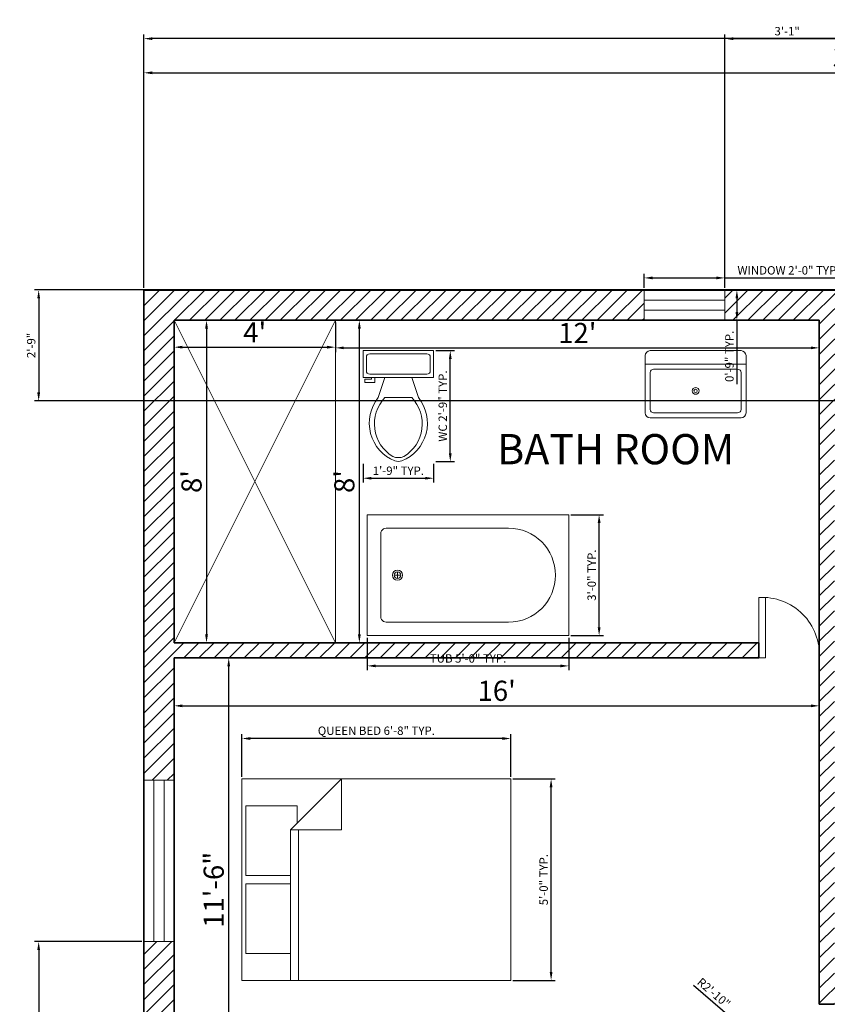
# Model space of a CAD drawing. Units: inches. Extents: x 4740 to 5323, y 7115 to 7713.
# Tile 3 of 6: x 4740 to 4980, y 7420 to 7713. Entities that reach past the tile are written whole.
import ezdxf

# ---------------------------------------------------------------- set-up
doc = ezdxf.new("R2010")
doc.units = ezdxf.units.IN
for name, color, linetype, lineweight in [('A-ANNO-DIMS', 2, 'Continuous', 18), ('A-AREA-IDEN', 7, 'Continuous', 25), ('A-DOOR', 4, 'Continuous', 18), ('A-FLOR-FIXT', 9, 'Continuous', 18), ('A-FURN', 8, 'Continuous', 18), ('A-GLAZ', 242, 'Continuous', 18), ('A-WALL', 7, 'Continuous', 35)]:
    doc.layers.add(name, color=color, linetype=linetype, lineweight=lineweight)
doc.layers.add('A-WALL-PATT', color=152, linetype='Continuous', lineweight=13, true_color=0x2776bb)
doc.styles.get("Standard").update_dxf_attribs({"font": 'arial.ttf'})
doc.dimstyles.new('ISO-25', dxfattribs={"dimtxt": 2.5, "dimasz": 2.5, "dimexe": 1.25, "dimexo": 0.625, "dimtad": 1, "dimlunit": 3, "dimtxsty": 'Standard', "dimcen": 2.5, "dimadec": 0, "dimazin": 0, "dimtfac": 1, "dimtmove": 0, "dimatfit": 3, "dimfxl": 1, "dimarcsym": 0})

# ---------------------------------------------------------------- blocks, each defined once
blk = doc.blocks.new('*D11')
at = {"layer": 'A-ANNO-DIMS', "color": 0, "lineweight": -2, "transparency": 16777216}
for p, q in [((4785.46, 7622.73), (4785.46, 7614.09)), ((4833.46, 7622.73), (4833.46, 7614.09)), ((4787.96, 7615.34), (4830.96, 7615.34))]:
    blk.add_line(p, q, dxfattribs=at)
at = {"layer": 'A-ANNO-DIMS', "color": 0, "transparency": 16777216}
for points in [[(4787.96, 7615.76), (4787.96, 7614.92), (4785.46, 7615.34)], [(4830.96, 7615.76), (4830.96, 7614.92), (4833.46, 7615.34)]]:
    blk.add_solid(points, dxfattribs=at)
at = {"layer": 'Defpoints', "color": 0, "transparency": 16777216}
for p in [(4785.46, 7623.36), (4833.46, 7623.36), (4833.46, 7615.34)]:
    blk.add_point(p, dxfattribs=at)
at = {"layer": 'A-ANNO-DIMS', "color": 0, "transparency": 16777216, "insert": (4809.46, 7618.97), "char_height": 6, "attachment_point": 5}
blk.add_mtext("4'", dxfattribs=at)
blk = doc.blocks.new('*D12')
at = {"layer": 'A-ANNO-DIMS', "color": 0, "lineweight": -2, "transparency": 16777216}
for p, q in [((4786.08, 7623.36), (4796.37, 7623.36)), ((4795.12, 7620.86), (4795.12, 7529.86)), ((4786.08, 7527.36), (4796.37, 7527.36))]:
    blk.add_line(p, q, dxfattribs=at)
at = {"layer": 'A-ANNO-DIMS', "color": 0, "transparency": 16777216}
for points in [[(4794.7, 7620.86), (4795.54, 7620.86), (4795.12, 7623.36)], [(4794.7, 7529.86), (4795.54, 7529.86), (4795.12, 7527.36)]]:
    blk.add_solid(points, dxfattribs=at)
at = {"layer": 'Defpoints', "color": 0, "transparency": 16777216}
for p in [(4785.46, 7623.36), (4785.46, 7527.36), (4795.12, 7527.36)]:
    blk.add_point(p, dxfattribs=at)
at = {"layer": 'A-ANNO-DIMS', "color": 0, "transparency": 16777216, "insert": (4791.43, 7575.36), "char_height": 6, "attachment_point": 5, "rotation": 90}
blk.add_mtext("8'", dxfattribs=at)
blk = doc.blocks.new('*D13')
at = {"layer": 'A-ANNO-DIMS', "color": 0, "lineweight": -2, "transparency": 16777216}
for p, q in [((4834.08, 7623.36), (4841.84, 7623.36)), ((4840.59, 7529.86), (4840.59, 7620.86)), ((4834.08, 7527.36), (4841.84, 7527.36))]:
    blk.add_line(p, q, dxfattribs=at)
at = {"layer": 'A-ANNO-DIMS', "color": 0, "transparency": 16777216}
for points in [[(4840.18, 7620.86), (4841.01, 7620.86), (4840.59, 7623.36)], [(4840.18, 7529.86), (4841.01, 7529.86), (4840.59, 7527.36)]]:
    blk.add_solid(points, dxfattribs=at)
at = {"layer": 'Defpoints', "color": 0, "transparency": 16777216}
for p in [(4833.46, 7623.36), (4840.59, 7623.36), (4833.46, 7527.36)]:
    blk.add_point(p, dxfattribs=at)
at = {"layer": 'A-ANNO-DIMS', "color": 0, "transparency": 16777216, "insert": (4836.9, 7575.36), "char_height": 6, "attachment_point": 5, "rotation": 90}
blk.add_mtext("8'", dxfattribs=at)
blk = doc.blocks.new('*D14')
at = {"layer": 'A-ANNO-DIMS', "color": 0, "lineweight": -2, "transparency": 16777216}
for p, q in [((4833.46, 7622.73), (4833.46, 7613.89)), ((4977.46, 7622.73), (4977.46, 7613.89)), ((4835.96, 7615.14), (4974.96, 7615.14))]:
    blk.add_line(p, q, dxfattribs=at)
at = {"layer": 'A-ANNO-DIMS', "color": 0, "transparency": 16777216}
for points in [[(4835.96, 7615.55), (4835.96, 7614.72), (4833.46, 7615.14)], [(4974.96, 7615.55), (4974.96, 7614.72), (4977.46, 7615.14)]]:
    blk.add_solid(points, dxfattribs=at)
at = {"layer": 'Defpoints', "color": 0, "transparency": 16777216}
for p in [(4833.46, 7623.36), (4977.46, 7623.36), (4977.46, 7615.14)]:
    blk.add_point(p, dxfattribs=at)
at = {"layer": 'A-ANNO-DIMS', "color": 0, "transparency": 16777216, "insert": (4905.46, 7618.77), "char_height": 6, "width": 4.0075, "attachment_point": 5}
blk.add_mtext("12'", dxfattribs=at)
blk = doc.blocks.new('*D15')
at = {"layer": 'A-ANNO-DIMS', "color": 0, "lineweight": -2, "transparency": 16777216}
for p, q in [((4785.46, 7522.23), (4785.46, 7507.36)), ((4977.46, 7522.23), (4977.46, 7507.36)), ((4787.96, 7508.61), (4974.96, 7508.61))]:
    blk.add_line(p, q, dxfattribs=at)
at = {"layer": 'A-ANNO-DIMS', "color": 0, "transparency": 16777216}
for points in [[(4787.96, 7509.02), (4787.96, 7508.19), (4785.46, 7508.61)], [(4974.96, 7509.02), (4974.96, 7508.19), (4977.46, 7508.61)]]:
    blk.add_solid(points, dxfattribs=at)
at = {"layer": 'Defpoints', "color": 0, "transparency": 16777216}
for p in [(4785.46, 7522.86), (4977.46, 7522.86), (4977.46, 7508.61)]:
    blk.add_point(p, dxfattribs=at)
at = {"layer": 'A-ANNO-DIMS', "color": 0, "transparency": 16777216, "insert": (4881.46, 7512.3), "char_height": 6, "attachment_point": 5}
blk.add_mtext("16'", dxfattribs=at)
blk = doc.blocks.new('*D16')
at = {"layer": 'A-ANNO-DIMS', "color": 0, "lineweight": -2, "transparency": 16777216}
for p, q in [((4786.08, 7522.86), (4802.97, 7522.86)), ((4801.72, 7387.36), (4801.72, 7520.36)), ((4786.08, 7384.86), (4802.97, 7384.86))]:
    blk.add_line(p, q, dxfattribs=at)
at = {"layer": 'A-ANNO-DIMS', "color": 0, "transparency": 16777216}
for points in [[(4801.3, 7520.36), (4802.13, 7520.36), (4801.72, 7522.86)], [(4801.3, 7387.36), (4802.13, 7387.36), (4801.72, 7384.86)]]:
    blk.add_solid(points, dxfattribs=at)
at = {"layer": 'Defpoints', "color": 0, "transparency": 16777216}
for p in [(4785.46, 7522.86), (4801.72, 7522.86), (4785.46, 7384.86)]:
    blk.add_point(p, dxfattribs=at)
at = {"layer": 'A-ANNO-DIMS', "color": 0, "transparency": 16777216, "insert": (4798.03, 7453.86), "char_height": 6, "attachment_point": 5, "rotation": 90}
blk.add_mtext('11\'-6"', dxfattribs=at)
blk = doc.blocks.new('Bath Tub - 26 x 60 in.')
for p, q in [((9, -17), (9, -19)), ((8, -18), (10, -18))]:
    blk.add_line(p, q)
blk.add_lwpolyline([(0, -36), (0, 0), (60, 0), (60, -36)], close=True)
for points in [[(6, -4), (42, -4)], [(4, -30), (4, -6)], [(42, -32), (6, -32)]]:
    blk.add_lwpolyline(points)
for radius in [1.5, 1]:
    blk.add_circle((9, -18), radius)
for centre, radius, start, end in [((5.75, -5.75), 1.77, 81.8699, 188.1301), ((42, -18), 14, 270, 90), ((5.75, -30.25), 1.77, 171.8699, 278.1301)]:
    blk.add_arc(centre, radius, start, end)
blk = doc.blocks.new('Toilet - top')
for p, q in [((9.5, -6), (9.5, -2)), ((-10, -8.5), (-8, -8.5)), ((-10, -9.5), (-10, -8.5)), ((-8, -8.5), (-8, -8)), ((-7, -8), (-7, -9.5)), ((-4, -8), (-6, -14)), ((4, -8), (6, -14)), ((-7, -9.5), (-10, -9.5)), ((4, -14), (-4, -14))]:
    blk.add_line(p, q)
blk.add_lwpolyline([(10.5, -8), (10.5, 0), (-10.5, 0), (-10.5, -8)], close=True)
for points in [[(-9.5, -2), (-9.5, -6)], [(8.5, -1), (-8.5, -1)], [(-8.5, -7), (8.5, -7)]]:
    blk.add_lwpolyline(points)
for centre, radius, start, end in [((-8.62, -1.88), 0.884, 81.8699, 188.1301), ((8.62, -1.88), 0.884, 351.8699, 98.1301), ((-8.62, -6.12), 0.884, 171.8699, 278.1301), ((8.62, -6.12), 0.884, 261.8699, 8.1301), ((3.52, -21.58), 12.17, 141.4691, 247.9714), ((4.2, -21.82), 11.33, 136.3677, 238.9468), ((-3.52, -21.58), 12.17, 292.0284, 38.5307), ((-4.2, -21.82), 11.33, 301.053, 43.6321), ((0, -27.88), 4, 245.7318, 294.2682), ((0, -29), 4, 254.8605, 285.1395)]:
    blk.add_arc(centre, radius, start, end)
blk = doc.blocks.new('Bed - Queen')
for p, q in [((0, -80.00003), (0, 0)), ((0, 0), (59.99999, 0)), ((59.99999, 0), (59.99999, -80.00003)), ((7.99999, -1.2), (28.79998, -1.2)), ((7.99999, -14.4), (7.99999, -1.2)), ((28.79998, -1.2), (28.79998, -14.4)), ((31.19999, -1.2), (51.99999, -1.2)), ((31.19999, -14.4), (31.19999, -1.2)), ((51.99999, -1.2), (51.99999, -16.4)), ((0, -14.4), (44.8, -14.4)), ((59.99999, -29.6), (44.8, -14.4)), ((44.8, -14.4), (44.8, -29.6)), ((44.8, -16.8), (0, -16.8)), ((51.99999, -16.4), (46.79936, -16.4)), ((44.8, -29.6), (59.99999, -29.6)), ((59.99999, -80.00003), (0, -80.00003))]:
    blk.add_line(p, q)
blk = doc.blocks.new('Sink-single - 30 in top')
blk.add_line((-15, -3.999996), (15, -3.999996))
for points in [[(-13.5, 0), (13.5, 0)], [(-15, -18.499996), (-15, -1.5)], [(15, -1.5), (15, -18.499996)], [(-12.5, -5.499996), (12.5, -5.499996)], [(-13.5, -17.499996), (-13.5, -6.499996)], [(13.5, -6.499996), (13.5, -17.499996)], [(13.5, -19.999996), (-13.5, -19.999996)], [(12.5, -18.499996), (-12.5, -18.499996)]]:
    blk.add_lwpolyline(points)
for radius in [1, 0.5]:
    blk.add_circle((0, -11.999996), radius)
for centre, radius, start, end in [((-13.5, -1.5), 1.5, 90, 180), ((13.5, -1.5), 1.5, 0, 90), ((-12.5, -6.499996), 1, 90, 180), ((12.5, -6.499996), 1, 0, 90), ((-12.5, -17.499996), 1, 180, 270), ((12.5, -17.499996), 1, 270, 0), ((-13.5, -18.499996), 1.5, 180, 270), ((13.5, -18.499996), 1.5, 270, 0)]:
    blk.add_arc(centre, radius, start, end)
blk = doc.blocks.new('*D35')
at = {"layer": 'A-ANNO-DIMS', "color": 0, "lineweight": -2, "transparency": 16777216}
for p, q in [((4776.46, 7632.98), (4776.46, 7698.25)), ((5215.96, 7629.25), (5215.96, 7698.25)), ((4778.96, 7697), (5213.46, 7697))]:
    blk.add_line(p, q, dxfattribs=at)
at = {"layer": 'A-ANNO-DIMS', "color": 0, "transparency": 16777216}
for points in [[(4778.96, 7697.42), (4778.96, 7696.58), (4776.46, 7697)], [(5213.46, 7697.42), (5213.46, 7696.58), (5215.96, 7697)]]:
    blk.add_solid(points, dxfattribs=at)
at = {"layer": 'Defpoints', "color": 0, "transparency": 16777216}
for p in [(5215.96, 7697), (4776.46, 7632.36), (5215.96, 7628.62)]:
    blk.add_point(p, dxfattribs=at)
at = {"layer": 'A-ANNO-DIMS', "color": 0, "transparency": 16777216, "insert": (4996.21, 7700.69), "char_height": 6, "attachment_point": 5}
blk.add_mtext('36\'-7.5"', dxfattribs=at)
blk = doc.blocks.new('WIN-48IN')
for p, q in [((0, 0), (0, 9)), ((0, 9), (48, 9)), ((48, 9), (48, 0)), ((0, 6), (48, 6)), ((0, 3), (48, 3)), ((48, 0), (0, 0))]:
    blk.add_line(p, q)
blk = doc.blocks.new('WIN-24IN')
for p, q in [((0, 24), (9, 24)), ((0, 24), (0, 0)), ((3, 0), (3, 24)), ((6, 0), (6, 24)), ((9, 0), (9, 24)), ((0, 0), (9, 0))]:
    blk.add_line(p, q)
blk = doc.blocks.new('DOOR-SWING-18IN')
for p, q in [((0, 0), (0, 18)), ((0, 18), (2, 18)), ((2, 18), (2, 0)), ((2, 0), (0, 0))]:
    blk.add_line(p, q)
blk.add_arc((1, 1), 17.03, 356.6335, 93.3665)
blk = doc.blocks.new('*D44')
at = {"layer": 'A-ANNO-DIMS', "color": 0, "lineweight": -2, "transparency": 16777216}
for p, q in [((4925.34, 7632.98), (4925.34, 7637.21)), ((4949.34, 7632.98), (4949.34, 7637.21)), ((4927.84, 7635.96), (4946.84, 7635.96)), ((4949.34, 7635.96), (4984.73, 7635.96))]:
    blk.add_line(p, q, dxfattribs=at)
at = {"layer": 'A-ANNO-DIMS', "color": 0, "transparency": 16777216}
for points in [[(4927.84, 7636.37), (4927.84, 7635.54), (4925.34, 7635.96)], [(4946.84, 7636.37), (4946.84, 7635.54), (4949.34, 7635.96)]]:
    blk.add_solid(points, dxfattribs=at)
at = {"layer": 'Defpoints', "color": 0, "transparency": 16777216}
for p in [(4949.34, 7635.96), (4925.34, 7632.36), (4949.34, 7632.36)]:
    blk.add_point(p, dxfattribs=at)
at = {"layer": 'A-ANNO-DIMS', "color": 0, "transparency": 16777216, "insert": (4968.29, 7637.88), "char_height": 2.5, "attachment_point": 5}
blk.add_mtext('WINDOW 2\'-0" TYP.', dxfattribs=at)
blk = doc.blocks.new('*D45')
at = {"layer": 'A-ANNO-DIMS', "color": 0, "lineweight": -2, "transparency": 16777216}
for p, q in [((4949.97, 7632.36), (4954.19, 7632.36)), ((4952.94, 7629.86), (4952.94, 7625.86)), ((4949.97, 7623.36), (4954.19, 7623.36)), ((4952.94, 7623.36), (4952.94, 7604.37))]:
    blk.add_line(p, q, dxfattribs=at)
at = {"layer": 'A-ANNO-DIMS', "color": 0, "transparency": 16777216}
for points in [[(4952.53, 7629.86), (4953.36, 7629.86), (4952.94, 7632.36)], [(4952.53, 7625.86), (4953.36, 7625.86), (4952.94, 7623.36)]]:
    blk.add_solid(points, dxfattribs=at)
at = {"layer": 'Defpoints', "color": 0, "transparency": 16777216}
for p in [(4949.34, 7632.36), (4949.34, 7623.36), (4952.94, 7623.36)]:
    blk.add_point(p, dxfattribs=at)
at = {"layer": 'A-ANNO-DIMS', "color": 0, "transparency": 16777216, "insert": (4951.04, 7612.61), "char_height": 2.5, "attachment_point": 5, "rotation": 90}
blk.add_mtext('0\'-9" TYP.', dxfattribs=at)
blk = doc.blocks.new('*D48')
at = {"layer": 'A-ANNO-DIMS', "color": 0, "lineweight": -2, "transparency": 16777216}
for p, q in [((4842.95, 7528.86), (4842.95, 7519.24)), ((4902.95, 7528.86), (4902.95, 7519.24)), ((4845.45, 7520.49), (4900.45, 7520.49))]:
    blk.add_line(p, q, dxfattribs=at)
at = {"layer": 'A-ANNO-DIMS', "color": 0, "transparency": 16777216}
for points in [[(4845.45, 7520.9), (4845.45, 7520.07), (4842.95, 7520.49)], [(4900.45, 7520.9), (4900.45, 7520.07), (4902.95, 7520.49)]]:
    blk.add_solid(points, dxfattribs=at)
at = {"layer": 'Defpoints', "color": 0, "transparency": 16777216}
for p in [(4842.95, 7529.49), (4902.95, 7529.49), (4902.95, 7520.49)]:
    blk.add_point(p, dxfattribs=at)
at = {"layer": 'A-ANNO-DIMS', "color": 0, "transparency": 16777216, "insert": (4872.95, 7522.39), "char_height": 2.5, "attachment_point": 5}
blk.add_mtext('TUB 5\'-0" TYP.', dxfattribs=at)
blk = doc.blocks.new('*D49')
at = {"layer": 'A-ANNO-DIMS', "color": 0, "lineweight": -2, "transparency": 16777216}
for p, q in [((4903.57, 7565.49), (4913.2, 7565.49)), ((4911.95, 7531.99), (4911.95, 7562.99)), ((4903.57, 7529.49), (4913.2, 7529.49))]:
    blk.add_line(p, q, dxfattribs=at)
at = {"layer": 'A-ANNO-DIMS', "color": 0, "transparency": 16777216}
for points in [[(4911.53, 7562.99), (4912.37, 7562.99), (4911.95, 7565.49)], [(4911.53, 7531.99), (4912.37, 7531.99), (4911.95, 7529.49)]]:
    blk.add_solid(points, dxfattribs=at)
at = {"layer": 'Defpoints', "color": 0, "transparency": 16777216}
for p in [(4902.95, 7565.49), (4911.95, 7565.49), (4902.95, 7529.49)]:
    blk.add_point(p, dxfattribs=at)
at = {"layer": 'A-ANNO-DIMS', "color": 0, "transparency": 16777216, "insert": (4910.05, 7547.49), "char_height": 2.5, "attachment_point": 5, "rotation": 90}
blk.add_mtext('3\'-0" TYP.', dxfattribs=at)
blk = doc.blocks.new('*D50')
at = {"layer": 'A-ANNO-DIMS', "color": 0, "lineweight": -2, "transparency": 16777216}
for p, q in [((4805.65, 7487.5), (4805.65, 7500.13)), ((4883.16, 7498.88), (4808.15, 7498.88)), ((4885.66, 7487.5), (4885.66, 7500.13))]:
    blk.add_line(p, q, dxfattribs=at)
at = {"layer": 'A-ANNO-DIMS', "color": 0, "transparency": 16777216}
for points in [[(4808.15, 7499.29), (4808.15, 7498.46), (4805.65, 7498.88)], [(4883.16, 7499.29), (4883.16, 7498.46), (4885.66, 7498.88)]]:
    blk.add_solid(points, dxfattribs=at)
at = {"layer": 'Defpoints', "color": 0, "transparency": 16777216}
for p in [(4805.65, 7498.88), (4805.65, 7486.88), (4885.66, 7486.88)]:
    blk.add_point(p, dxfattribs=at)
at = {"layer": 'A-ANNO-DIMS', "color": 0, "transparency": 16777216, "insert": (4845.65, 7500.87), "char_height": 2.5, "attachment_point": 5}
blk.add_mtext('QUEEN BED 6\'-8" TYP.', dxfattribs=at)
blk = doc.blocks.new('*D51')
at = {"layer": 'A-ANNO-DIMS', "color": 0, "lineweight": -2, "transparency": 16777216}
for p, q in [((4886.28, 7486.88), (4898.91, 7486.88)), ((4897.66, 7429.38), (4897.66, 7484.38)), ((4886.28, 7426.88), (4898.91, 7426.88))]:
    blk.add_line(p, q, dxfattribs=at)
at = {"layer": 'A-ANNO-DIMS', "color": 0, "transparency": 16777216}
for points in [[(4897.24, 7484.38), (4898.07, 7484.38), (4897.66, 7486.88)], [(4897.24, 7429.38), (4898.07, 7429.38), (4897.66, 7426.88)]]:
    blk.add_solid(points, dxfattribs=at)
at = {"layer": 'Defpoints', "color": 0, "transparency": 16777216}
for p in [(4885.66, 7486.88), (4897.66, 7486.88), (4885.66, 7426.88)]:
    blk.add_point(p, dxfattribs=at)
at = {"layer": 'A-ANNO-DIMS', "color": 0, "transparency": 16777216, "insert": (4895.75, 7456.88), "char_height": 2.5, "attachment_point": 5, "rotation": 90}
blk.add_mtext('5\'-0" TYP.', dxfattribs=at)
blk = doc.blocks.new('*D52')
at = {"layer": 'A-ANNO-DIMS', "color": 0, "lineweight": -2, "transparency": 16777216}
for p, q in [((4863.32, 7614.34), (4868.9, 7614.34)), ((4867.65, 7583.79), (4867.65, 7611.84)), ((4863.32, 7581.29), (4868.9, 7581.29))]:
    blk.add_line(p, q, dxfattribs=at)
at = {"layer": 'A-ANNO-DIMS', "color": 0, "transparency": 16777216}
for points in [[(4867.24, 7611.84), (4868.07, 7611.84), (4867.65, 7614.34)], [(4867.24, 7583.79), (4868.07, 7583.79), (4867.65, 7581.29)]]:
    blk.add_solid(points, dxfattribs=at)
at = {"layer": 'Defpoints', "color": 0, "transparency": 16777216}
for p in [(4862.7, 7614.34), (4867.65, 7614.34), (4862.7, 7581.29)]:
    blk.add_point(p, dxfattribs=at)
at = {"layer": 'A-ANNO-DIMS', "color": 0, "transparency": 16777216, "insert": (4865.74, 7597.82), "char_height": 2.5, "attachment_point": 5, "rotation": 90}
blk.add_mtext('WC 2\'-9" TYP.', dxfattribs=at)
blk = doc.blocks.new('*D53')
at = {"layer": 'A-ANNO-DIMS', "color": 0, "lineweight": -2, "transparency": 16777216}
for p, q in [((4841.7, 7580.67), (4841.7, 7575.09)), ((4862.7, 7580.67), (4862.7, 7575.09)), ((4844.2, 7576.34), (4860.2, 7576.34))]:
    blk.add_line(p, q, dxfattribs=at)
at = {"layer": 'A-ANNO-DIMS', "color": 0, "transparency": 16777216}
for points in [[(4844.2, 7576.75), (4844.2, 7575.92), (4841.7, 7576.34)], [(4860.2, 7576.75), (4860.2, 7575.92), (4862.7, 7576.34)]]:
    blk.add_solid(points, dxfattribs=at)
at = {"layer": 'Defpoints', "color": 0, "transparency": 16777216}
for p in [(4841.7, 7581.29), (4862.7, 7581.29), (4862.7, 7576.34)]:
    blk.add_point(p, dxfattribs=at)
at = {"layer": 'A-ANNO-DIMS', "color": 0, "transparency": 16777216, "insert": (4852.2, 7578.24), "char_height": 2.5, "attachment_point": 5}
blk.add_mtext('1\'-9" TYP.', dxfattribs=at)
blk = doc.blocks.new('*D73')
at = {"layer": 'A-ANNO-DIMS', "color": 0, "lineweight": -2, "transparency": 16777216}
for p, q in [((4775.83, 7438.45), (4743.91, 7438.45)), ((4745.16, 7435.95), (4745.16, 7378.36)), ((4775.83, 7375.86), (4743.91, 7375.86))]:
    blk.add_line(p, q, dxfattribs=at)
at = {"layer": 'A-ANNO-DIMS', "color": 0, "transparency": 16777216}
for points in [[(4744.74, 7435.95), (4745.58, 7435.95), (4745.16, 7438.45)], [(4744.74, 7378.36), (4745.58, 7378.36), (4745.16, 7375.86)]]:
    blk.add_solid(points, dxfattribs=at)
at = {"layer": 'Defpoints', "color": 0, "transparency": 16777216}
for p in [(4776.46, 7438.45), (4745.16, 7375.86), (4776.46, 7375.86)]:
    blk.add_point(p, dxfattribs=at)
at = {"layer": 'A-ANNO-DIMS', "color": 0, "transparency": 16777216, "insert": (4743.24, 7407.15), "char_height": 2.5, "attachment_point": 5, "rotation": 90}
blk.add_mtext('5\'-2 1/2"', dxfattribs=at)
blk = doc.blocks.new('*D74')
at = {"layer": 'A-ANNO-DIMS', "color": 0, "lineweight": -2, "transparency": 16777216}
for p, q in [((4949.34, 7632.98), (4949.34, 7708.41)), ((4951.84, 7707.16), (4983.96, 7707.16)), ((4986.46, 7632.98), (4986.46, 7708.41))]:
    blk.add_line(p, q, dxfattribs=at)
at = {"layer": 'A-ANNO-DIMS', "color": 0, "transparency": 16777216}
for points in [[(4951.84, 7707.57), (4951.84, 7706.74), (4949.34, 7707.16)], [(4983.96, 7707.57), (4983.96, 7706.74), (4986.46, 7707.16)]]:
    blk.add_solid(points, dxfattribs=at)
at = {"layer": 'Defpoints', "color": 0, "transparency": 16777216}
for p in [(4986.46, 7707.16), (4949.34, 7632.36), (4986.46, 7632.36)]:
    blk.add_point(p, dxfattribs=at)
at = {"layer": 'A-ANNO-DIMS', "color": 0, "transparency": 16777216, "insert": (4967.9, 7709.06), "char_height": 2.5, "attachment_point": 5}
blk.add_mtext('3\'-1"', dxfattribs=at)
blk = doc.blocks.new('*D81')
at = {"layer": 'A-ANNO-DIMS', "color": 0, "lineweight": -2, "transparency": 16777216}
for p, q in [((4776.46, 7632.98), (4776.46, 7708.41)), ((5264.46, 7707.16), (4778.96, 7707.16)), ((5266.96, 7422.98), (5266.96, 7708.41))]:
    blk.add_line(p, q, dxfattribs=at)
at = {"layer": 'A-ANNO-DIMS', "color": 0, "transparency": 16777216}
for points in [[(4778.96, 7707.57), (4778.96, 7706.74), (4776.46, 7707.16)], [(5264.46, 7707.57), (5264.46, 7706.74), (5266.96, 7707.16)]]:
    blk.add_solid(points, dxfattribs=at)
at = {"layer": 'Defpoints', "color": 0, "transparency": 16777216}
for p in [(4776.46, 7707.16), (4776.46, 7632.36), (5266.96, 7422.36)]:
    blk.add_point(p, dxfattribs=at)
at = {"layer": 'A-ANNO-DIMS', "color": 0, "transparency": 16777216, "insert": (5021.71, 7709.07), "char_height": 2.5, "attachment_point": 5}
blk.add_mtext('40\'-10 1/2"', dxfattribs=at)
blk = doc.blocks.new('*D82')
at = {"layer": 'A-ANNO-DIMS', "color": 0, "lineweight": -2, "transparency": 16777216}
for p, q in [((4985.83, 7632.36), (4743.91, 7632.36)), ((4745.16, 7629.86), (4745.16, 7601.86)), ((4985.83, 7599.36), (4743.91, 7599.36))]:
    blk.add_line(p, q, dxfattribs=at)
at = {"layer": 'A-ANNO-DIMS', "color": 0, "transparency": 16777216}
for points in [[(4744.74, 7629.86), (4745.58, 7629.86), (4745.16, 7632.36)], [(4744.74, 7601.86), (4745.58, 7601.86), (4745.16, 7599.36)]]:
    blk.add_solid(points, dxfattribs=at)
at = {"layer": 'Defpoints', "color": 0, "transparency": 16777216}
for p in [(4986.46, 7632.36), (4745.16, 7599.36), (4986.46, 7599.36)]:
    blk.add_point(p, dxfattribs=at)
at = {"layer": 'A-ANNO-DIMS', "color": 0, "transparency": 16777216, "insert": (4743.26, 7615.86), "char_height": 2.5, "attachment_point": 5, "rotation": 90}
blk.add_mtext('2\'-9"', dxfattribs=at)
blk = doc.blocks.new('*D90')
at = {"layer": 'A-ANNO-DIMS', "color": 0, "lineweight": -2, "transparency": 16777216}
for p, q in [((4940.01, 7425.47), (4958.3, 7409.76)), ((4986.12, 7385.86), (4960.2, 7408.13))]:
    blk.add_line(p, q, dxfattribs=at)
at = {"layer": 'A-ANNO-DIMS', "color": 0, "transparency": 16777216}
blk.add_solid([(4958.57, 7410.07), (4958.03, 7409.44), (4960.2, 7408.13)], dxfattribs=at)
at = {"layer": 'Defpoints', "color": 0, "transparency": 16777216}
for p in [(4960.2, 7408.13), (4986.12, 7385.86)]:
    blk.add_point(p, dxfattribs=at)
at = {"layer": 'A-ANNO-DIMS', "color": 0, "transparency": 16777216, "insert": (4945.88, 7422.93), "char_height": 2.5, "attachment_point": 5, "rotation": 319.334}
blk.add_mtext('R2\'-10"', dxfattribs=at)

msp = doc.modelspace()

# ---------------------------------------------------------------- hatches: boundary and pattern name
at = {"layer": 'A-WALL-PATT'}
h = msp.add_hatch(dxfattribs=at)
h.set_pattern_fill('ANSI31', color=256)
h.paths.add_polyline_path([(4925.343, 7632.357), (4776.459, 7632.357), (4776.459, 7486.448), (4785.459, 7486.448), (4785.459, 7522.857), (4959.459, 7522.857), (4959.459, 7527.357), (4785.459, 7527.357), (4785.459, 7623.357), (4833.459, 7623.357), (4925.343, 7623.357)])
h.paths.add_polyline_path([(5010.258, 7599.357), (5004.258, 7599.357), (4986.459, 7599.357), (4986.459, 7623.357), (4986.459, 7632.357), (4977.459, 7632.357), (4949.343, 7632.357), (4949.343, 7623.357), (4977.459, 7623.357), (4977.459, 7599.357), (4977.459, 7594.857), (4977.459, 7590.357), (4977.459, 7524.857, -0.0293864), (4977.459, 7522.857), (4977.459, 7426.857), (4977.459, 7422.357), (4977.459, 7419.778), (4981.959, 7419.778), (4981.959, 7422.357), (5041.959, 7422.357), (5041.959, 7479.357), (5037.459, 7479.357), (5037.459, 7426.857), (4981.959, 7426.857), (4981.959, 7590.357), (5010.258, 7590.357)])
h.paths.add_polyline_path([(5086.959, 7666.857), (5206.959, 7666.857), (5206.959, 7646.624), (5215.959, 7646.624), (5215.959, 7675.857), (5077.959, 7675.857), (5077.959, 7599.357), (5046.258, 7599.357), (5046.258, 7590.357), (5082.459, 7590.357), (5082.459, 7474.857, -0.0106371), (5084.459, 7474.857), (5086.959, 7474.857)])
h.paths.add_polyline_path([(5215.959, 7610.624), (5206.959, 7610.624), (5206.959, 7594.857), (5104.959, 7594.857), (5104.959, 7592.357, -0.0293864), (5104.959, 7590.357), (5206.959, 7590.357), (5206.959, 7426.857), (5104.959, 7426.857), (5082.459, 7426.857), (5082.459, 7422.357), (5104.959, 7422.357), (5215.959, 7422.357), (5215.959, 7464.357), (5215.959, 7506.357)])
h.paths.add_polyline_path([(4881.459, 7375.857), (4977.459, 7375.857), (4977.459, 7296.657), (4981.959, 7296.657), (4981.959, 7384.857), (4951.959, 7384.857), (4785.459, 7384.857), (4785.459, 7438.448), (4776.459, 7438.448), (4776.459, 7375.857), (4872.459, 7375.857), (4872.459, 7337.044), (4881.459, 7337.044)])
h.paths.add_polyline_path([(4881.459, 7313.044), (4872.459, 7313.044), (4872.459, 7148.157), (4916.568, 7148.157), (4916.568, 7157.157), (4881.459, 7157.157), (4881.459, 7269.357), (4981.959, 7269.357), (4981.959, 7273.857), (4963.959, 7273.857), (4881.459, 7273.857)])
h.paths.add_polyline_path([(5029.959, 7296.657), (5116.509, 7296.657), (5116.509, 7299.157, -0.0121933), (5116.509, 7301.157), (5025.459, 7301.157), (5025.459, 7157.157), (4964.568, 7157.157), (4964.568, 7148.157), (5076.933, 7148.157), (5076.933, 7157.157), (5029.959, 7157.157)])
h.paths.add_polyline_path([(5182.959, 7203.442), (5173.959, 7203.442), (5173.959, 7157.157), (5124.933, 7157.157), (5124.933, 7148.157), (5182.959, 7148.157)])
h.paths.add_polyline_path([(5266.959, 7353.764), (5257.959, 7353.764), (5257.959, 7301.157), (5182.959, 7301.157), (5158.509, 7301.157), (5158.509, 7296.657), (5173.959, 7296.657), (5173.959, 7263.442), (5182.959, 7263.442), (5182.959, 7292.157), (5266.959, 7292.157)])
h.paths.add_polyline_path([(5266.959, 7422.357), (5257.959, 7422.357), (5257.959, 7377.764), (5266.959, 7377.764)])

# ---------------------------------------------------------------- linework, layer by layer
at = {"layer": 'A-FLOR-FIXT'}
for p, q in [((4785.459, 7527.357), (4833.459, 7623.357)), ((4833.459, 7623.357), (4785.459, 7623.357)), ((4785.459, 7623.357), (4833.459, 7527.357)), ((4833.459, 7623.357), (4833.459, 7527.357)), ((4833.459, 7527.357), (4785.459, 7527.357))]:
    msp.add_line(p, q, dxfattribs=at)
at = {"layer": 'A-WALL'}
for p, q in [((4977.459, 7632.357), (4776.459, 7632.357)), ((4776.459, 7375.857), (4776.459, 7632.357)), ((4977.459, 7632.357), (4986.459, 7632.357)), ((4977.459, 7623.357), (4785.459, 7623.357)), ((4785.459, 7623.357), (4785.459, 7527.357)), ((4977.459, 7599.357), (4977.459, 7623.357)), ((4977.459, 7594.857), (4977.459, 7599.357)), ((4977.459, 7594.857), (4977.459, 7590.357)), ((4977.459, 7590.357), (4977.459, 7426.857)), ((4959.459, 7527.357), (4785.459, 7527.357)), ((4959.459, 7527.357), (4959.459, 7522.857)), ((4959.459, 7522.857), (4785.459, 7522.857)), ((4785.459, 7522.857), (4785.459, 7384.857)), ((4977.459, 7426.857), (4977.459, 7422.357)), ((4977.459, 7422.357), (4977.459, 7419.778)), ((4977.459, 7419.778), (4981.959, 7419.778))]:
    msp.add_line(p, q, dxfattribs=at)

# ---------------------------------------------------------------- block references
at = {"layer": 'A-DOOR'}
msp.add_blockref('DOOR-SWING-18IN', (4959.459, 7522.857), dxfattribs=at)
at = {"layer": 'A-FLOR-FIXT'}
for name, p in [('Toilet - top', (4852.198, 7614.34)), ('Sink-single - 30 in top', (4940.673, 7614.321)), ('Bath Tub - 26 x 60 in.', (4842.949, 7565.488))]:
    msp.add_blockref(name, p, dxfattribs=at)
at = {"layer": 'A-FURN', "rotation": 90}
msp.add_blockref('Bed - Queen', (4805.655, 7426.877), dxfattribs=at)
at = {"layer": 'A-GLAZ'}
for name, p, rotation in [('WIN-24IN', (4925.343, 7632.357), 270.0000000000038), ('WIN-48IN', (4785.459, 7438.448), 90.0000000000021)]:
    msp.add_blockref(name, p, dxfattribs=dict(at, rotation=rotation))

# ---------------------------------------------------------------- texts
at = {"layer": 'A-AREA-IDEN', "insert": (4881.602, 7589.491), "char_height": 9, "attachment_point": 1}
msp.add_mtext_dynamic_manual_height_columns('{BATH ROOM}', width=75.84022, gutter_width=12.5, heights=[0], dxfattribs=at)

# ---------------------------------------------------------------- dimensions: what is measured, and where the dimension line sits
at = {"layer": 'A-ANNO-DIMS'}
for base, p1, p2, override, picture, middle in [((4776.459, 7707.157), (5266.959, 7422.357), (4776.459, 7632.357), {"dimdec": 1, "dimlfac": 1, "dimrnd": 0, "dimzin": 1, "dimdsep": 46, "dimlunit": 4, "dimfrac": 2}, '*D81', (5021.709, 7709.074)), ((4986.459, 7707.157), (4949.343, 7632.357), (4986.459, 7632.357), {"dimdec": 1, "dimlfac": 1, "dimrnd": 0, "dimzin": 1, "dimdsep": 46, "dimlunit": 4, "dimfrac": 2}, '*D74', (4967.901, 7709.059)), ((5215.959, 7697.001), (4776.459, 7632.357), (5215.959, 7628.624), {"dimtxt": 6, "dimclrd": 0, "dimclre": 0, "dimclrt": 0}, '*D35', (4996.209, 7700.692)), ((4833.459, 7615.34), (4785.459, 7623.357), (4833.459, 7623.357), {"dimtxt": 6, "dimclrd": 0, "dimclre": 0, "dimclrt": 0}, '*D11', (4809.459, 7618.965)), ((4977.459, 7615.136), (4833.459, 7623.357), (4977.459, 7623.357), {"dimtxt": 6, "dimclrd": 0, "dimclre": 0, "dimclrt": 0}, '*D14', (4905.459, 7618.774)), ((4977.459, 7508.607), (4785.459, 7522.857), (4977.459, 7522.857), {"dimtxt": 6, "dimclrd": 0, "dimclre": 0, "dimclrt": 0}, '*D15', (4881.459, 7512.295))]:
    dim = msp.add_linear_dim(base=base, p1=p1, p2=p2, dimstyle='ISO-25', override=override, dxfattribs=at)
    dim.commit()
    dim.dimension.update_dxf_attribs({"geometry": picture, "text_midpoint": middle})
for base, p1, p2, angle, text, picture, middle in [((4949.343, 7635.957), (4925.343, 7632.357), (4949.343, 7632.357), 0, 'WINDOW <> TYP.', '*D44', (4968.286, 7637.875)), ((4952.943, 7623.357), (4949.343, 7632.357), (4949.343, 7623.357), 270, '<> TYP.', '*D45', (4951.042, 7612.612)), ((4867.655, 7614.34), (4862.698, 7581.293), (4862.698, 7614.34), 90, 'WC <> TYP.', '*D52', (4865.737, 7597.816)), ((4911.949, 7565.488), (4902.949, 7529.488), (4902.949, 7565.488), 90, '<> TYP.', '*D49', (4910.047, 7547.488)), ((4805.655, 7498.877), (4885.655, 7486.877), (4805.655, 7486.877), 180, 'QUEEN BED <> TYP.', '*D50', (4845.655, 7500.872)), ((4897.655, 7486.877), (4885.655, 7426.877), (4885.655, 7486.877), 90, '<> TYP.', '*D51', (4895.754, 7456.877))]:
    dim = msp.add_linear_dim(base=base, p1=p1, p2=p2, angle=angle, text=text, dimstyle='ISO-25', override={"dimdec": 1, "dimlfac": 1, "dimrnd": 0, "dimzin": 1, "dimdsep": 46, "dimlunit": 4, "dimfrac": 2}, dxfattribs=at)
    dim.commit()
    dim.dimension.update_dxf_attribs({"geometry": picture, "text_midpoint": middle})
for base, p1, p2, override, picture, middle in [((4745.159, 7599.357), (4986.459, 7632.357), (4986.459, 7599.357), {"dimdec": 1, "dimlfac": 1, "dimrnd": 0, "dimzin": 1, "dimdsep": 46, "dimlunit": 4, "dimfrac": 2}, '*D82', (4743.258, 7615.857)), ((4795.12, 7527.357), (4785.459, 7623.357), (4785.459, 7527.357), {"dimtxt": 6, "dimclrd": 0, "dimclre": 0, "dimclrt": 0}, '*D12', (4791.432, 7575.357)), ((4840.592, 7623.357), (4833.459, 7527.357), (4833.459, 7623.357), {"dimtxt": 6, "dimclrd": 0, "dimclre": 0, "dimclrt": 0}, '*D13', (4836.904, 7575.357)), ((4801.718, 7522.857), (4785.459, 7384.857), (4785.459, 7522.857), {"dimtxt": 6, "dimclrd": 0, "dimclre": 0, "dimclrt": 0}, '*D16', (4798.029, 7453.857)), ((4745.159, 7375.857), (4776.459, 7438.448), (4776.459, 7375.857), {"dimdec": 1, "dimlfac": 1, "dimrnd": 0, "dimzin": 1, "dimdsep": 46, "dimlunit": 4, "dimfrac": 2}, '*D73', (4743.242, 7407.152))]:
    dim = msp.add_linear_dim(base=base, p1=p1, p2=p2, angle=90, dimstyle='ISO-25', override=override, dxfattribs=at)
    dim.commit()
    dim.dimension.update_dxf_attribs({"geometry": picture, "text_midpoint": middle})
for base, p1, p2, text, picture, middle in [((4862.698, 7576.336), (4841.698, 7581.293), (4862.698, 7581.293), '<> TYP.', '*D53', (4852.198, 7578.238)), ((4902.949, 7520.488), (4842.949, 7529.488), (4902.949, 7529.488), 'TUB <> TYP.', '*D48', (4872.949, 7522.389))]:
    dim = msp.add_linear_dim(base=base, p1=p1, p2=p2, text=text, dimstyle='ISO-25', override={"dimdec": 1, "dimlfac": 1, "dimrnd": 0, "dimzin": 1, "dimdsep": 46, "dimlunit": 4, "dimfrac": 2}, dxfattribs=at)
    dim.commit()
    dim.dimension.update_dxf_attribs({"geometry": picture, "text_midpoint": middle})
dim = msp.add_radius_dim(center=(4986.12, 7385.857), mpoint=(4960.197, 7408.127), dimstyle='ISO-25', override={"dimdec": 1, "dimlfac": 1, "dimrnd": 0, "dimzin": 1, "dimdsep": 46, "dimlunit": 4, "dimfrac": 2}, dxfattribs=at)
dim.commit()
dim.dimension.update_dxf_attribs({"geometry": '*D90', "text_midpoint": (4944.644, 7421.489), "dimtype": 164})

doc.saveas('drawing.dxf')
